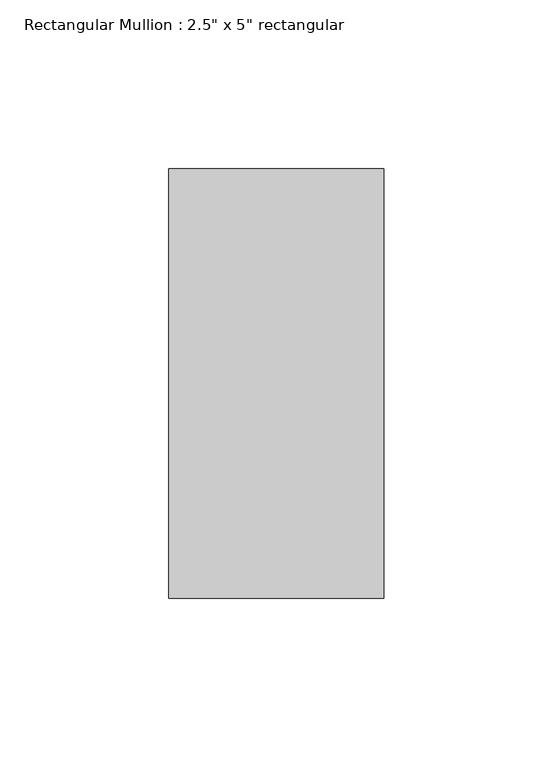
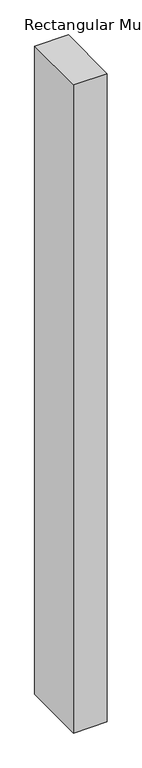
"""IFC4 building model written with IfcOpenShell, lengths in millimetres: member geometry."""

from ifc_helpers import new_model, si_unit, frame, origin, place, context, project, spatial, polyline, outline, extrude, source, transform, mapped, element, save


def member_15f4dda0(model_context):
    return source(origin(), model_context, "Body", "SweptSolid", [
        extrude(outline(polyline([(31.75, 63.5), (31.75, -63.5), (-31.75, -63.5), (-31.75, 63.5), (31.75, 63.5)])), frame((0.0, 0.0, -1293.8688597), z_axis=(0.0, 0.0, 1.0), x_axis=(1.0, 0.0, 0.0)), (0.0, 0.0, 1.0), 1293.8688597),
    ])


if __name__ == "__main__":
    model = new_model("IFC4")
    model_context = context("Model", 3, world=origin())
    ifc_project = project(units=[si_unit("LENGTHUNIT", "METRE", prefix="MILLI")], contexts=[model_context])
    site = spatial("IfcSite", under=ifc_project)
    building = spatial("IfcBuilding", under=site)
    placement = place(None, origin())
    member_shape = member_15f4dda0(model_context)
    element("IfcMember", 1, ObjectType="Rectangular Mullion : 2.5\" x 5\" rectangular", at=placement, inside=building, context=model_context, shape_type="MappedRepresentation", body=[
        mapped(member_shape, transform((0.0, 0.0, 0.0), x_axis=(1.0, 0.0, 0.0), y_axis=(0.0, 1.0, 0.0), z_axis=(0.0, 0.0, 1.0))),
    ])
    save(model, "model.ifc")

# Revit data of these elements
# Type "Rectangular Mullion : 2.5\" x 5\" rectangular"
#   built-in parameter 1007304 = 0.416667 (stored number, unit not read)
#   built-in parameter 1007301 = 0.104167 (stored number, unit not read)
#   built-in parameter 1007300 = 0.104167 (stored number, unit not read)
# Element 1 (IfcMember, "Rectangular Mullion : 2.5\" x 5\" rectangular")
#   Materials on its faces: "metal black"
# Materials
#   "metal black": class "Generic", colour RGB 120 120 120, transparency 0, Cost = 0
